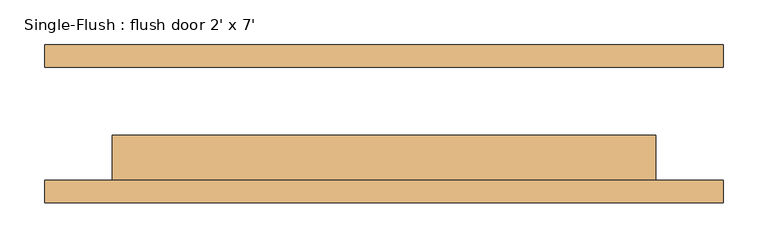
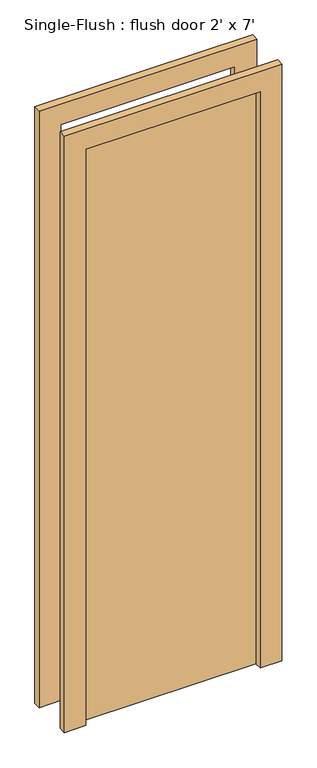
"""IFC4 building model written with IfcOpenShell, lengths in millimetres: door geometry, Single-Flush : flush door 2' x 7'."""

from ifc_helpers import new_model, si_unit, frame, origin, origin_with_axes, place, context, project, spatial, polyline, outline, extrude, source, transform, mapped, element, save


def single_flush_flush_door_2_x_7_931cabab(model_context):
    return source(origin(), model_context, "Body", "SweptSolid", [
        extrude(outline(polyline([(2209.8, -381.0), (0.0, -381.0), (0.0, -304.8), (2133.6, -304.8), (2133.6, 304.8), (0.0, 304.8), (0.0, 381.0), (2209.8, 381.0), (2209.8, -381.0)])), frame((0.0, -88.9, 0.0), z_axis=(0.0, 1.0, 0.0), x_axis=(0.0, 0.0, 1.0)), (0.0, 0.0, 1.0), 25.4),
        extrude(outline(polyline([(2209.8, 381.0), (2209.8, -381.0), (0.0, -381.0), (0.0, -304.8), (2133.6, -304.8), (2133.6, 304.8), (0.0, 304.8), (0.0, 381.0), (2209.8, 381.0)])), frame((0.0, 63.5, 0.0), z_axis=(0.0, 1.0, 0.0), x_axis=(0.0, 0.0, 1.0)), (0.0, 0.0, 1.0), 25.4),
        extrude(outline(polyline([(304.8, -12.7), (304.8, -63.5), (-304.8, -63.5), (-304.8, -12.7), (304.8, -12.7)])), origin_with_axes(), (0.0, 0.0, 1.0), 2133.6),
    ])


if __name__ == "__main__":
    model = new_model("IFC4")
    model_context = context("Model", 3, world=origin())
    ifc_project = project(units=[si_unit("LENGTHUNIT", "METRE", prefix="MILLI")], contexts=[model_context])
    site = spatial("IfcSite", under=ifc_project)
    building = spatial("IfcBuilding", under=site)
    placement = place(None, origin())
    single_flush_flush_door_2_x_7_shape = single_flush_flush_door_2_x_7_931cabab(model_context)
    element("IfcDoor", 1, ObjectType="Single-Flush : flush door 2' x 7'", at=placement, inside=building, context=model_context, shape_type="MappedRepresentation", body=[
        mapped(single_flush_flush_door_2_x_7_shape, transform((0.0, 0.0, 0.0), x_axis=(1.0, 0.0, 0.0), y_axis=(0.0, 1.0, 0.0), z_axis=(0.0, 0.0, 1.0))),
    ])
    save(model, "model.ifc")

# Revit data of these elements
# Type "Single-Flush : flush door 2' x 7'"
#   Type Mark = "12"
#   Construction Type Id = "MDOOR"
#   Assembly Code = "C1020"
#   Analytic Construction = "Metal"
#   Thickness = 0' - 2"
#   Heat Transfer Coefficient (U) = 0.651978 BTU/(h·ft²·°F)
#   Height = 7' - 0"
#   Trim Projection Ext = 0' - 1"
#   Trim Projection Int = 0' - 1"
#   Trim Width = 0' - 3"
#   Width = 2' - 0"
#   Define Thermal Properties by = 1
#   Door Material = Door - Panel
#   Frame Material = Door - Frame
#   Visual Light Transmittance = 0
#   Solar Heat Gain Coefficient = 0
#   Function = (empty or 0)
#   Wall Closure = (empty or 0)
# Element 1 (IfcDoor, "Single-Flush : flush door 2' x 7'")
#   Materials on its faces: "Door - Frame", "Door - Panel"
# Materials
#   "Door - Panel": class "Wood", colour RGB 210 159 95, transparency 0, Cost = 0
#   "Door - Frame": colour RGB 118 70 51, transparency 0, Cost = 0
